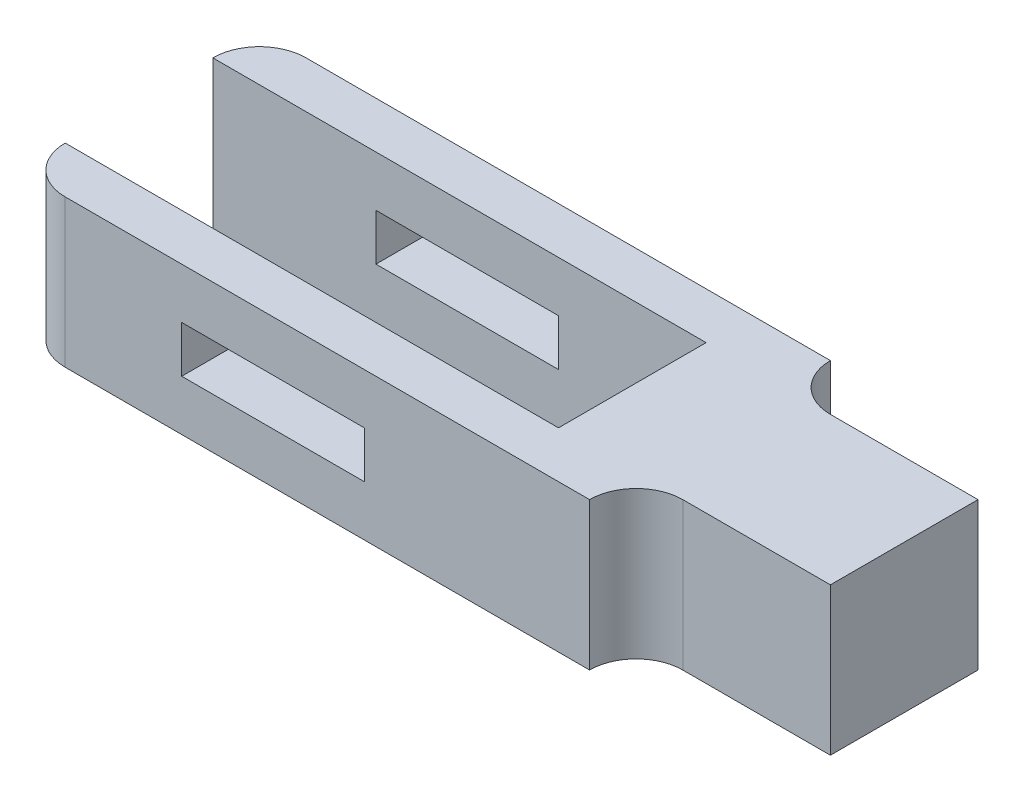
ISO-10303-21;
HEADER;
FILE_DESCRIPTION(('STEP AP214'),'2;1');
FILE_NAME('part.step','',(''),(''),'','','');
FILE_SCHEMA(('AUTOMOTIVE_DESIGN { 1 0 10303 214 1 1 1 1 }'));
ENDSEC;
DATA;
#1=APPLICATION_CONTEXT('core data for automotive mechanical design processes');
#2=APPLICATION_PROTOCOL_DEFINITION('international standard','automotive_design',2000,#1);
#3=PRODUCT_CONTEXT('',#1,'mechanical');
#4=PRODUCT('Part','Part','',(#3));
#5=PRODUCT_RELATED_PRODUCT_CATEGORY('part','',(#4));
#6=PRODUCT_DEFINITION_FORMATION('','',#4);
#7=PRODUCT_DEFINITION_CONTEXT('part definition',#1,'design');
#8=PRODUCT_DEFINITION('design','',#6,#7);
#9=PRODUCT_DEFINITION_SHAPE('','',#8);
#10=(LENGTH_UNIT() NAMED_UNIT(*) SI_UNIT(.MILLI.,.METRE.));
#11=(NAMED_UNIT(*) PLANE_ANGLE_UNIT() SI_UNIT($,.RADIAN.));
#12=(NAMED_UNIT(*) SI_UNIT($,.STERADIAN.) SOLID_ANGLE_UNIT());
#13=UNCERTAINTY_MEASURE_WITH_UNIT(LENGTH_MEASURE(1.E-05),#10,'distance_accuracy_value','');
#14=(GEOMETRIC_REPRESENTATION_CONTEXT(3) GLOBAL_UNCERTAINTY_ASSIGNED_CONTEXT((#13)) GLOBAL_UNIT_ASSIGNED_CONTEXT((#10,
#11,#12)) REPRESENTATION_CONTEXT('',''));
#15=CARTESIAN_POINT('',(0.,0.,0.));
#16=DIRECTION('',(0.,0.,1.));
#17=DIRECTION('',(1.,0.,0.));
#18=AXIS2_PLACEMENT_3D('',#15,#16,#17);
#19=CARTESIAN_POINT('',(-137.,38.,-31.));
#20=DIRECTION('',(0.,0.,1.));
#21=DIRECTION('',(1.,0.,0.));
#22=AXIS2_PLACEMENT_3D('',#19,#20,#21);
#23=PLANE('',#22);
#24=DIRECTION('',(1.,0.,0.));
#25=VECTOR('',#24,1.);
#26=CARTESIAN_POINT('',(-137.,13.,-31.));
#27=LINE('',#26,#25);
#28=CARTESIAN_POINT('',(-95.,13.,-31.));
#29=VERTEX_POINT('',#28);
#30=CARTESIAN_POINT('',(-48.,13.,-31.));
#31=VERTEX_POINT('',#30);
#32=EDGE_CURVE('E233',#29,#31,#27,.T.);
#33=ORIENTED_EDGE('',*,*,#32,.T.);
#34=DIRECTION('',(0.,1.,0.));
#35=VECTOR('',#34,1.);
#36=CARTESIAN_POINT('',(-48.,38.,-31.));
#37=LINE('',#36,#35);
#38=CARTESIAN_POINT('',(-48.,25.,-31.));
#39=VERTEX_POINT('',#38);
#40=EDGE_CURVE('E244',#31,#39,#37,.T.);
#41=ORIENTED_EDGE('',*,*,#40,.T.);
#42=DIRECTION('',(-1.,0.,0.));
#43=VECTOR('',#42,1.);
#44=CARTESIAN_POINT('',(-137.,25.,-31.));
#45=LINE('',#44,#43);
#46=CARTESIAN_POINT('',(-95.,25.,-31.));
#47=VERTEX_POINT('',#46);
#48=EDGE_CURVE('E218',#39,#47,#45,.T.);
#49=ORIENTED_EDGE('',*,*,#48,.T.);
#50=DIRECTION('',(0.,-1.,0.));
#51=VECTOR('',#50,1.);
#52=CARTESIAN_POINT('',(-95.,38.,-31.));
#53=LINE('',#52,#51);
#54=EDGE_CURVE('E227',#47,#29,#53,.T.);
#55=ORIENTED_EDGE('',*,*,#54,.T.);
#56=EDGE_LOOP('',(#33,#41,#49,#55));
#57=FACE_BOUND('',#56,.T.);
#58=DIRECTION('',(-1.,0.,0.));
#59=VECTOR('',#58,1.);
#60=CARTESIAN_POINT('',(-137.,0.,-31.));
#61=LINE('',#60,#59);
#62=CARTESIAN_POINT('',(10.,0.,-31.));
#63=VERTEX_POINT('',#62);
#64=CARTESIAN_POINT('',(-125.,0.,-31.));
#65=VERTEX_POINT('',#64);
#66=EDGE_CURVE('E268',#63,#65,#61,.T.);
#67=ORIENTED_EDGE('',*,*,#66,.T.);
#68=DIRECTION('',(0.,-1.,0.));
#69=VECTOR('',#68,1.);
#70=CARTESIAN_POINT('',(-125.,38.,-31.));
#71=LINE('',#70,#69);
#72=CARTESIAN_POINT('',(-125.,38.,-31.));
#73=VERTEX_POINT('',#72);
#74=EDGE_CURVE('E11',#65,#73,#71,.F.);
#75=ORIENTED_EDGE('',*,*,#74,.T.);
#76=DIRECTION('',(-1.,0.,0.));
#77=VECTOR('',#76,1.);
#78=CARTESIAN_POINT('',(-10.,38.,-31.));
#79=LINE('',#78,#77);
#80=CARTESIAN_POINT('',(10.,38.,-31.));
#81=VERTEX_POINT('',#80);
#82=EDGE_CURVE('E267',#81,#73,#79,.T.);
#83=ORIENTED_EDGE('',*,*,#82,.F.);
#84=DIRECTION('',(0.,-1.,0.));
#85=VECTOR('',#84,1.);
#86=CARTESIAN_POINT('',(10.,38.,-31.));
#87=LINE('',#86,#85);
#88=EDGE_CURVE('E301',#81,#63,#87,.T.);
#89=ORIENTED_EDGE('',*,*,#88,.T.);
#90=EDGE_LOOP('',(#67,#75,#83,#89));
#91=FACE_BOUND('',#90,.T.);
#92=ADVANCED_FACE('F39',(#57,#91),#23,.F.);
#93=CARTESIAN_POINT('',(-10.,38.,-19.));
#94=DIRECTION('',(0.,0.,-1.));
#95=DIRECTION('',(-1.,0.,0.));
#96=AXIS2_PLACEMENT_3D('',#93,#94,#95);
#97=PLANE('',#96);
#98=DIRECTION('',(1.,0.,0.));
#99=VECTOR('',#98,1.);
#100=CARTESIAN_POINT('',(-10.,25.,-19.));
#101=LINE('',#100,#99);
#102=CARTESIAN_POINT('',(-95.,25.,-19.));
#103=VERTEX_POINT('',#102);
#104=CARTESIAN_POINT('',(-48.,25.,-19.));
#105=VERTEX_POINT('',#104);
#106=EDGE_CURVE('E216',#103,#105,#101,.T.);
#107=ORIENTED_EDGE('',*,*,#106,.T.);
#108=DIRECTION('',(0.,-1.,0.));
#109=VECTOR('',#108,1.);
#110=CARTESIAN_POINT('',(-48.,38.,-19.));
#111=LINE('',#110,#109);
#112=CARTESIAN_POINT('',(-48.,13.,-19.));
#113=VERTEX_POINT('',#112);
#114=EDGE_CURVE('E242',#105,#113,#111,.T.);
#115=ORIENTED_EDGE('',*,*,#114,.T.);
#116=DIRECTION('',(-1.,0.,0.));
#117=VECTOR('',#116,1.);
#118=CARTESIAN_POINT('',(-10.,13.,-19.));
#119=LINE('',#118,#117);
#120=CARTESIAN_POINT('',(-95.,13.,-19.));
#121=VERTEX_POINT('',#120);
#122=EDGE_CURVE('E234',#113,#121,#119,.T.);
#123=ORIENTED_EDGE('',*,*,#122,.T.);
#124=DIRECTION('',(0.,1.,0.));
#125=VECTOR('',#124,1.);
#126=CARTESIAN_POINT('',(-95.,38.,-19.));
#127=LINE('',#126,#125);
#128=EDGE_CURVE('E224',#121,#103,#127,.T.);
#129=ORIENTED_EDGE('',*,*,#128,.T.);
#130=EDGE_LOOP('',(#107,#115,#123,#129));
#131=FACE_BOUND('',#130,.T.);
#132=DIRECTION('',(1.,0.,0.));
#133=VECTOR('',#132,1.);
#134=CARTESIAN_POINT('',(-10.,0.,-19.));
#135=LINE('',#134,#133);
#136=CARTESIAN_POINT('',(-137.,0.,-19.));
#137=VERTEX_POINT('',#136);
#138=CARTESIAN_POINT('',(-10.,0.,-19.));
#139=VERTEX_POINT('',#138);
#140=EDGE_CURVE('E285',#137,#139,#135,.T.);
#141=ORIENTED_EDGE('',*,*,#140,.T.);
#142=DIRECTION('',(0.,-1.,0.));
#143=VECTOR('',#142,1.);
#144=CARTESIAN_POINT('',(-10.,38.,-19.));
#145=LINE('',#144,#143);
#146=CARTESIAN_POINT('',(-10.,38.,-19.));
#147=VERTEX_POINT('',#146);
#148=EDGE_CURVE('E298',#147,#139,#145,.T.);
#149=ORIENTED_EDGE('',*,*,#148,.F.);
#150=DIRECTION('',(1.,0.,0.));
#151=VECTOR('',#150,1.);
#152=CARTESIAN_POINT('',(-10.,38.,-19.));
#153=LINE('',#152,#151);
#154=CARTESIAN_POINT('',(-137.,38.,-19.));
#155=VERTEX_POINT('',#154);
#156=EDGE_CURVE('E271',#155,#147,#153,.T.);
#157=ORIENTED_EDGE('',*,*,#156,.F.);
#158=DIRECTION('',(0.,-1.,0.));
#159=VECTOR('',#158,1.);
#160=CARTESIAN_POINT('',(-137.,38.,-19.));
#161=LINE('',#160,#159);
#162=EDGE_CURVE('E302',#155,#137,#161,.T.);
#163=ORIENTED_EDGE('',*,*,#162,.T.);
#164=EDGE_LOOP('',(#141,#149,#157,#163));
#165=FACE_BOUND('',#164,.T.);
#166=ADVANCED_FACE('F355',(#131,#165),#97,.F.);
#167=CARTESIAN_POINT('',(-10.,38.,19.));
#168=DIRECTION('',(1.,0.,0.));
#169=DIRECTION('',(0.,0.,-1.));
#170=AXIS2_PLACEMENT_3D('',#167,#168,#169);
#171=PLANE('',#170);
#172=DIRECTION('',(0.,0.,1.));
#173=VECTOR('',#172,1.);
#174=CARTESIAN_POINT('',(-10.,0.,19.));
#175=LINE('',#174,#173);
#176=CARTESIAN_POINT('',(-10.,0.,19.));
#177=VERTEX_POINT('',#176);
#178=EDGE_CURVE('E284',#139,#177,#175,.T.);
#179=ORIENTED_EDGE('',*,*,#178,.T.);
#180=DIRECTION('',(0.,-1.,0.));
#181=VECTOR('',#180,1.);
#182=CARTESIAN_POINT('',(-10.,38.,19.));
#183=LINE('',#182,#181);
#184=CARTESIAN_POINT('',(-10.,38.,19.));
#185=VERTEX_POINT('',#184);
#186=EDGE_CURVE('E293',#185,#177,#183,.T.);
#187=ORIENTED_EDGE('',*,*,#186,.F.);
#188=DIRECTION('',(0.,0.,1.));
#189=VECTOR('',#188,1.);
#190=CARTESIAN_POINT('',(-10.,38.,19.));
#191=LINE('',#190,#189);
#192=EDGE_CURVE('E273',#147,#185,#191,.T.);
#193=ORIENTED_EDGE('',*,*,#192,.F.);
#194=ORIENTED_EDGE('',*,*,#148,.T.);
#195=EDGE_LOOP('',(#179,#187,#193,#194));
#196=FACE_BOUND('',#195,.T.);
#197=ADVANCED_FACE('F349',(#196),#171,.F.);
#198=CARTESIAN_POINT('',(-137.,38.,19.));
#199=DIRECTION('',(0.,0.,1.));
#200=DIRECTION('',(1.,0.,0.));
#201=AXIS2_PLACEMENT_3D('',#198,#199,#200);
#202=PLANE('',#201);
#203=DIRECTION('',(1.,0.,0.));
#204=VECTOR('',#203,1.);
#205=CARTESIAN_POINT('',(-137.,13.,19.));
#206=LINE('',#205,#204);
#207=CARTESIAN_POINT('',(-95.,13.,19.));
#208=VERTEX_POINT('',#207);
#209=CARTESIAN_POINT('',(-48.,13.,19.));
#210=VERTEX_POINT('',#209);
#211=EDGE_CURVE('E229',#208,#210,#206,.T.);
#212=ORIENTED_EDGE('',*,*,#211,.T.);
#213=DIRECTION('',(0.,1.,0.));
#214=VECTOR('',#213,1.);
#215=CARTESIAN_POINT('',(-48.,38.,19.));
#216=LINE('',#215,#214);
#217=CARTESIAN_POINT('',(-48.,25.,19.));
#218=VERTEX_POINT('',#217);
#219=EDGE_CURVE('E236',#210,#218,#216,.T.);
#220=ORIENTED_EDGE('',*,*,#219,.T.);
#221=DIRECTION('',(-1.,0.,0.));
#222=VECTOR('',#221,1.);
#223=CARTESIAN_POINT('',(-137.,25.,19.));
#224=LINE('',#223,#222);
#225=CARTESIAN_POINT('',(-95.,25.,19.));
#226=VERTEX_POINT('',#225);
#227=EDGE_CURVE('E212',#218,#226,#224,.T.);
#228=ORIENTED_EDGE('',*,*,#227,.T.);
#229=DIRECTION('',(0.,-1.,0.));
#230=VECTOR('',#229,1.);
#231=CARTESIAN_POINT('',(-95.,38.,19.));
#232=LINE('',#231,#230);
#233=EDGE_CURVE('E181',#226,#208,#232,.T.);
#234=ORIENTED_EDGE('',*,*,#233,.T.);
#235=EDGE_LOOP('',(#212,#220,#228,#234));
#236=FACE_BOUND('',#235,.T.);
#237=DIRECTION('',(-1.,0.,0.));
#238=VECTOR('',#237,1.);
#239=CARTESIAN_POINT('',(-137.,0.,19.));
#240=LINE('',#239,#238);
#241=CARTESIAN_POINT('',(-137.,0.,19.));
#242=VERTEX_POINT('',#241);
#243=EDGE_CURVE('E287',#177,#242,#240,.T.);
#244=ORIENTED_EDGE('',*,*,#243,.T.);
#245=DIRECTION('',(0.,-1.,0.));
#246=VECTOR('',#245,1.);
#247=CARTESIAN_POINT('',(-137.,38.,19.));
#248=LINE('',#247,#246);
#249=CARTESIAN_POINT('',(-137.,38.,19.));
#250=VERTEX_POINT('',#249);
#251=EDGE_CURVE('E295',#250,#242,#248,.T.);
#252=ORIENTED_EDGE('',*,*,#251,.F.);
#253=DIRECTION('',(-1.,0.,0.));
#254=VECTOR('',#253,1.);
#255=CARTESIAN_POINT('',(-137.,38.,19.));
#256=LINE('',#255,#254);
#257=EDGE_CURVE('E277',#185,#250,#256,.T.);
#258=ORIENTED_EDGE('',*,*,#257,.F.);
#259=ORIENTED_EDGE('',*,*,#186,.T.);
#260=EDGE_LOOP('',(#244,#252,#258,#259));
#261=FACE_BOUND('',#260,.T.);
#262=ADVANCED_FACE('F343',(#236,#261),#202,.F.);
#263=CARTESIAN_POINT('',(-10.,38.,31.));
#264=DIRECTION('',(0.,0.,-1.));
#265=DIRECTION('',(-1.,0.,0.));
#266=AXIS2_PLACEMENT_3D('',#263,#264,#265);
#267=PLANE('',#266);
#268=DIRECTION('',(-1.,0.,0.));
#269=VECTOR('',#268,1.);
#270=CARTESIAN_POINT('',(-95.,25.,31.));
#271=LINE('',#270,#269);
#272=CARTESIAN_POINT('',(-48.,25.,31.));
#273=VERTEX_POINT('',#272);
#274=CARTESIAN_POINT('',(-95.,25.,31.));
#275=VERTEX_POINT('',#274);
#276=EDGE_CURVE('E192',#273,#275,#271,.T.);
#277=ORIENTED_EDGE('',*,*,#276,.F.);
#278=DIRECTION('',(0.,1.,0.));
#279=VECTOR('',#278,1.);
#280=CARTESIAN_POINT('',(-48.,13.,31.));
#281=LINE('',#280,#279);
#282=CARTESIAN_POINT('',(-48.,13.,31.));
#283=VERTEX_POINT('',#282);
#284=EDGE_CURVE('E197',#283,#273,#281,.T.);
#285=ORIENTED_EDGE('',*,*,#284,.F.);
#286=DIRECTION('',(1.,0.,0.));
#287=VECTOR('',#286,1.);
#288=CARTESIAN_POINT('',(-95.,13.,31.));
#289=LINE('',#288,#287);
#290=CARTESIAN_POINT('',(-95.,13.,31.));
#291=VERTEX_POINT('',#290);
#292=EDGE_CURVE('E205',#291,#283,#289,.T.);
#293=ORIENTED_EDGE('',*,*,#292,.F.);
#294=DIRECTION('',(0.,-1.,0.));
#295=VECTOR('',#294,1.);
#296=CARTESIAN_POINT('',(-95.,13.,31.));
#297=LINE('',#296,#295);
#298=EDGE_CURVE('E178',#275,#291,#297,.T.);
#299=ORIENTED_EDGE('',*,*,#298,.F.);
#300=EDGE_LOOP('',(#277,#285,#293,#299));
#301=FACE_BOUND('',#300,.T.);
#302=DIRECTION('',(1.,0.,0.));
#303=VECTOR('',#302,1.);
#304=CARTESIAN_POINT('',(-10.,38.,31.));
#305=LINE('',#304,#303);
#306=CARTESIAN_POINT('',(-125.,38.,31.));
#307=VERTEX_POINT('',#306);
#308=CARTESIAN_POINT('',(10.,38.,31.));
#309=VERTEX_POINT('',#308);
#310=EDGE_CURVE('E279',#307,#309,#305,.T.);
#311=ORIENTED_EDGE('',*,*,#310,.F.);
#312=DIRECTION('',(0.,-1.,0.));
#313=VECTOR('',#312,1.);
#314=CARTESIAN_POINT('',(-125.,38.,31.));
#315=LINE('',#314,#313);
#316=CARTESIAN_POINT('',(-125.,0.,31.));
#317=VERTEX_POINT('',#316);
#318=EDGE_CURVE('E325',#307,#317,#315,.T.);
#319=ORIENTED_EDGE('',*,*,#318,.T.);
#320=DIRECTION('',(1.,0.,0.));
#321=VECTOR('',#320,1.);
#322=CARTESIAN_POINT('',(-10.,0.,31.));
#323=LINE('',#322,#321);
#324=CARTESIAN_POINT('',(10.,0.,31.));
#325=VERTEX_POINT('',#324);
#326=EDGE_CURVE('E275',#317,#325,#323,.T.);
#327=ORIENTED_EDGE('',*,*,#326,.T.);
#328=DIRECTION('',(0.,-1.,0.));
#329=VECTOR('',#328,1.);
#330=CARTESIAN_POINT('',(10.,38.,31.));
#331=LINE('',#330,#329);
#332=EDGE_CURVE('E278',#309,#325,#331,.T.);
#333=ORIENTED_EDGE('',*,*,#332,.F.);
#334=EDGE_LOOP('',(#311,#319,#327,#333));
#335=FACE_BOUND('',#334,.T.);
#336=ADVANCED_FACE('F200',(#301,#335),#267,.F.);
#337=CARTESIAN_POINT('',(0.,38.,0.));
#338=DIRECTION('',(0.,-1.,0.));
#339=DIRECTION('',(0.,0.,-1.));
#340=AXIS2_PLACEMENT_3D('',#337,#338,#339);
#341=PLANE('',#340);
#342=ORIENTED_EDGE('',*,*,#257,.T.);
#343=CARTESIAN_POINT('',(-125.,38.,19.));
#344=DIRECTION('',(0.,-1.,0.));
#345=DIRECTION('',(0.,0.,-1.));
#346=AXIS2_PLACEMENT_3D('',#343,#344,#345);
#347=CIRCLE('',#346,12.);
#348=EDGE_CURVE('E50',#250,#307,#347,.F.);
#349=ORIENTED_EDGE('',*,*,#348,.T.);
#350=ORIENTED_EDGE('',*,*,#310,.T.);
#351=CARTESIAN_POINT('',(22.,38.,31.));
#352=DIRECTION('',(0.,-1.,0.));
#353=DIRECTION('',(0.,0.,-1.));
#354=AXIS2_PLACEMENT_3D('',#351,#352,#353);
#355=CIRCLE('',#354,12.);
#356=CARTESIAN_POINT('',(22.,38.,19.));
#357=VERTEX_POINT('',#356);
#358=EDGE_CURVE('E316',#309,#357,#355,.T.);
#359=ORIENTED_EDGE('',*,*,#358,.T.);
#360=DIRECTION('',(-1.,0.,0.));
#361=VECTOR('',#360,1.);
#362=CARTESIAN_POINT('',(60.,38.,19.));
#363=LINE('',#362,#361);
#364=CARTESIAN_POINT('',(60.,38.,19.));
#365=VERTEX_POINT('',#364);
#366=EDGE_CURVE('E265',#365,#357,#363,.T.);
#367=ORIENTED_EDGE('',*,*,#366,.F.);
#368=DIRECTION('',(0.,0.,1.));
#369=VECTOR('',#368,1.);
#370=CARTESIAN_POINT('',(60.,38.,19.));
#371=LINE('',#370,#369);
#372=CARTESIAN_POINT('',(60.,38.,-19.));
#373=VERTEX_POINT('',#372);
#374=EDGE_CURVE('E248',#373,#365,#371,.T.);
#375=ORIENTED_EDGE('',*,*,#374,.F.);
#376=DIRECTION('',(-1.,0.,0.));
#377=VECTOR('',#376,1.);
#378=CARTESIAN_POINT('',(60.,38.,-19.));
#379=LINE('',#378,#377);
#380=CARTESIAN_POINT('',(22.,38.,-19.));
#381=VERTEX_POINT('',#380);
#382=EDGE_CURVE('E264',#373,#381,#379,.T.);
#383=ORIENTED_EDGE('',*,*,#382,.T.);
#384=CARTESIAN_POINT('',(22.,38.,-31.));
#385=DIRECTION('',(0.,-1.,0.));
#386=DIRECTION('',(0.,0.,-1.));
#387=AXIS2_PLACEMENT_3D('',#384,#385,#386);
#388=CIRCLE('',#387,12.);
#389=EDGE_CURVE('E318',#381,#81,#388,.T.);
#390=ORIENTED_EDGE('',*,*,#389,.T.);
#391=ORIENTED_EDGE('',*,*,#82,.T.);
#392=CARTESIAN_POINT('',(-125.,38.,-19.));
#393=DIRECTION('',(0.,-1.,0.));
#394=DIRECTION('',(0.,0.,-1.));
#395=AXIS2_PLACEMENT_3D('',#392,#393,#394);
#396=CIRCLE('',#395,12.);
#397=EDGE_CURVE('E327',#73,#155,#396,.F.);
#398=ORIENTED_EDGE('',*,*,#397,.T.);
#399=ORIENTED_EDGE('',*,*,#156,.T.);
#400=ORIENTED_EDGE('',*,*,#192,.T.);
#401=EDGE_LOOP('',(#342,#349,#350,#359,#367,#375,#383,#390,#391,#398,#399,#400));
#402=FACE_BOUND('',#401,.T.);
#403=ADVANCED_FACE('F335',(#402),#341,.F.);
#404=CARTESIAN_POINT('',(0.,0.,0.));
#405=DIRECTION('',(0.,-1.,0.));
#406=DIRECTION('',(0.,0.,-1.));
#407=AXIS2_PLACEMENT_3D('',#404,#405,#406);
#408=PLANE('',#407);
#409=ORIENTED_EDGE('',*,*,#326,.F.);
#410=CARTESIAN_POINT('',(-125.,0.,19.));
#411=DIRECTION('',(0.,-1.,0.));
#412=DIRECTION('',(0.,0.,-1.));
#413=AXIS2_PLACEMENT_3D('',#410,#411,#412);
#414=CIRCLE('',#413,12.);
#415=EDGE_CURVE('E326',#317,#242,#414,.T.);
#416=ORIENTED_EDGE('',*,*,#415,.T.);
#417=ORIENTED_EDGE('',*,*,#243,.F.);
#418=ORIENTED_EDGE('',*,*,#178,.F.);
#419=ORIENTED_EDGE('',*,*,#140,.F.);
#420=CARTESIAN_POINT('',(-125.,0.,-19.));
#421=DIRECTION('',(0.,-1.,0.));
#422=DIRECTION('',(0.,0.,-1.));
#423=AXIS2_PLACEMENT_3D('',#420,#421,#422);
#424=CIRCLE('',#423,12.);
#425=EDGE_CURVE('E58',#137,#65,#424,.T.);
#426=ORIENTED_EDGE('',*,*,#425,.T.);
#427=ORIENTED_EDGE('',*,*,#66,.F.);
#428=CARTESIAN_POINT('',(22.,0.,-31.));
#429=DIRECTION('',(0.,-1.,0.));
#430=DIRECTION('',(0.,0.,-1.));
#431=AXIS2_PLACEMENT_3D('',#428,#429,#430);
#432=CIRCLE('',#431,12.);
#433=CARTESIAN_POINT('',(22.,0.,-19.));
#434=VERTEX_POINT('',#433);
#435=EDGE_CURVE('E319',#63,#434,#432,.F.);
#436=ORIENTED_EDGE('',*,*,#435,.T.);
#437=DIRECTION('',(-1.,0.,0.));
#438=VECTOR('',#437,1.);
#439=CARTESIAN_POINT('',(60.,0.,-19.));
#440=LINE('',#439,#438);
#441=CARTESIAN_POINT('',(60.,0.,-19.));
#442=VERTEX_POINT('',#441);
#443=EDGE_CURVE('E258',#442,#434,#440,.T.);
#444=ORIENTED_EDGE('',*,*,#443,.F.);
#445=DIRECTION('',(0.,0.,-1.));
#446=VECTOR('',#445,1.);
#447=CARTESIAN_POINT('',(60.,0.,19.));
#448=LINE('',#447,#446);
#449=CARTESIAN_POINT('',(60.,0.,19.));
#450=VERTEX_POINT('',#449);
#451=EDGE_CURVE('E255',#450,#442,#448,.T.);
#452=ORIENTED_EDGE('',*,*,#451,.F.);
#453=DIRECTION('',(-1.,0.,0.));
#454=VECTOR('',#453,1.);
#455=CARTESIAN_POINT('',(60.,0.,19.));
#456=LINE('',#455,#454);
#457=CARTESIAN_POINT('',(22.,0.,19.));
#458=VERTEX_POINT('',#457);
#459=EDGE_CURVE('E259',#450,#458,#456,.T.);
#460=ORIENTED_EDGE('',*,*,#459,.T.);
#461=CARTESIAN_POINT('',(22.,0.,31.));
#462=DIRECTION('',(0.,-1.,0.));
#463=DIRECTION('',(0.,0.,-1.));
#464=AXIS2_PLACEMENT_3D('',#461,#462,#463);
#465=CIRCLE('',#464,12.);
#466=EDGE_CURVE('E311',#458,#325,#465,.F.);
#467=ORIENTED_EDGE('',*,*,#466,.T.);
#468=EDGE_LOOP('',(#409,#416,#417,#418,#419,#426,#427,#436,#444,#452,#460,#467));
#469=FACE_BOUND('',#468,.T.);
#470=ADVANCED_FACE('F344',(#469),#408,.T.);
#471=CARTESIAN_POINT('',(60.,0.,-19.));
#472=DIRECTION('',(0.,0.,1.));
#473=DIRECTION('',(1.,0.,0.));
#474=AXIS2_PLACEMENT_3D('',#471,#472,#473);
#475=PLANE('',#474);
#476=ORIENTED_EDGE('',*,*,#443,.T.);
#477=DIRECTION('',(0.,1.,0.));
#478=VECTOR('',#477,1.);
#479=CARTESIAN_POINT('',(22.,38.,-19.));
#480=LINE('',#479,#478);
#481=EDGE_CURVE('E309',#434,#381,#480,.T.);
#482=ORIENTED_EDGE('',*,*,#481,.T.);
#483=ORIENTED_EDGE('',*,*,#382,.F.);
#484=DIRECTION('',(0.,1.,0.));
#485=VECTOR('',#484,1.);
#486=CARTESIAN_POINT('',(60.,0.,-19.));
#487=LINE('',#486,#485);
#488=EDGE_CURVE('E249',#442,#373,#487,.T.);
#489=ORIENTED_EDGE('',*,*,#488,.F.);
#490=EDGE_LOOP('',(#476,#482,#483,#489));
#491=FACE_BOUND('',#490,.T.);
#492=ADVANCED_FACE('F368',(#491),#475,.F.);
#493=CARTESIAN_POINT('',(60.,0.,19.));
#494=DIRECTION('',(0.,0.,-1.));
#495=DIRECTION('',(-1.,0.,0.));
#496=AXIS2_PLACEMENT_3D('',#493,#494,#495);
#497=PLANE('',#496);
#498=ORIENTED_EDGE('',*,*,#366,.T.);
#499=DIRECTION('',(0.,-1.,0.));
#500=VECTOR('',#499,1.);
#501=CARTESIAN_POINT('',(22.,0.,19.));
#502=LINE('',#501,#500);
#503=EDGE_CURVE('E307',#357,#458,#502,.T.);
#504=ORIENTED_EDGE('',*,*,#503,.T.);
#505=ORIENTED_EDGE('',*,*,#459,.F.);
#506=DIRECTION('',(0.,-1.,0.));
#507=VECTOR('',#506,1.);
#508=CARTESIAN_POINT('',(60.,0.,19.));
#509=LINE('',#508,#507);
#510=EDGE_CURVE('E252',#365,#450,#509,.T.);
#511=ORIENTED_EDGE('',*,*,#510,.F.);
#512=EDGE_LOOP('',(#498,#504,#505,#511));
#513=FACE_BOUND('',#512,.T.);
#514=ADVANCED_FACE('F372',(#513),#497,.F.);
#515=CARTESIAN_POINT('',(60.,0.,0.));
#516=DIRECTION('',(-1.,0.,0.));
#517=DIRECTION('',(0.,0.,1.));
#518=AXIS2_PLACEMENT_3D('',#515,#516,#517);
#519=PLANE('',#518);
#520=ORIENTED_EDGE('',*,*,#488,.T.);
#521=ORIENTED_EDGE('',*,*,#374,.T.);
#522=ORIENTED_EDGE('',*,*,#510,.T.);
#523=ORIENTED_EDGE('',*,*,#451,.T.);
#524=EDGE_LOOP('',(#520,#521,#522,#523));
#525=FACE_BOUND('',#524,.T.);
#526=ADVANCED_FACE('F369',(#525),#519,.F.);
#527=CARTESIAN_POINT('',(-95.,25.,-53.));
#528=DIRECTION('',(0.,1.,0.));
#529=DIRECTION('',(0.,0.,1.));
#530=AXIS2_PLACEMENT_3D('',#527,#528,#529);
#531=PLANE('',#530);
#532=DIRECTION('',(0.,0.,1.));
#533=VECTOR('',#532,1.);
#534=CARTESIAN_POINT('',(-48.,25.,-53.));
#535=LINE('',#534,#533);
#536=EDGE_CURVE('E191',#218,#273,#535,.T.);
#537=ORIENTED_EDGE('',*,*,#536,.T.);
#538=ORIENTED_EDGE('',*,*,#276,.T.);
#539=DIRECTION('',(0.,0.,1.));
#540=VECTOR('',#539,1.);
#541=CARTESIAN_POINT('',(-95.,25.,-53.));
#542=LINE('',#541,#540);
#543=EDGE_CURVE('E171',#226,#275,#542,.T.);
#544=ORIENTED_EDGE('',*,*,#543,.F.);
#545=ORIENTED_EDGE('',*,*,#227,.F.);
#546=EDGE_LOOP('',(#537,#538,#544,#545));
#547=FACE_BOUND('',#546,.T.);
#548=ADVANCED_FACE('F194',(#547),#531,.F.);
#549=CARTESIAN_POINT('',(-95.,13.,-53.));
#550=DIRECTION('',(-1.,0.,0.));
#551=DIRECTION('',(0.,0.,1.));
#552=AXIS2_PLACEMENT_3D('',#549,#550,#551);
#553=PLANE('',#552);
#554=ORIENTED_EDGE('',*,*,#543,.T.);
#555=ORIENTED_EDGE('',*,*,#298,.T.);
#556=DIRECTION('',(0.,0.,1.));
#557=VECTOR('',#556,1.);
#558=CARTESIAN_POINT('',(-95.,13.,-53.));
#559=LINE('',#558,#557);
#560=EDGE_CURVE('E211',#208,#291,#559,.T.);
#561=ORIENTED_EDGE('',*,*,#560,.F.);
#562=ORIENTED_EDGE('',*,*,#233,.F.);
#563=EDGE_LOOP('',(#554,#555,#561,#562));
#564=FACE_BOUND('',#563,.T.);
#565=ADVANCED_FACE('F179',(#564),#553,.F.);
#566=CARTESIAN_POINT('',(-95.,13.,-53.));
#567=DIRECTION('',(0.,-1.,0.));
#568=DIRECTION('',(0.,0.,-1.));
#569=AXIS2_PLACEMENT_3D('',#566,#567,#568);
#570=PLANE('',#569);
#571=ORIENTED_EDGE('',*,*,#560,.T.);
#572=ORIENTED_EDGE('',*,*,#292,.T.);
#573=DIRECTION('',(0.,0.,1.));
#574=VECTOR('',#573,1.);
#575=CARTESIAN_POINT('',(-48.,13.,-53.));
#576=LINE('',#575,#574);
#577=EDGE_CURVE('E210',#210,#283,#576,.T.);
#578=ORIENTED_EDGE('',*,*,#577,.F.);
#579=ORIENTED_EDGE('',*,*,#211,.F.);
#580=EDGE_LOOP('',(#571,#572,#578,#579));
#581=FACE_BOUND('',#580,.T.);
#582=ADVANCED_FACE('F426',(#581),#570,.F.);
#583=CARTESIAN_POINT('',(-48.,13.,-53.));
#584=DIRECTION('',(1.,0.,0.));
#585=DIRECTION('',(0.,0.,-1.));
#586=AXIS2_PLACEMENT_3D('',#583,#584,#585);
#587=PLANE('',#586);
#588=ORIENTED_EDGE('',*,*,#577,.T.);
#589=ORIENTED_EDGE('',*,*,#284,.T.);
#590=ORIENTED_EDGE('',*,*,#536,.F.);
#591=ORIENTED_EDGE('',*,*,#219,.F.);
#592=EDGE_LOOP('',(#588,#589,#590,#591));
#593=FACE_BOUND('',#592,.T.);
#594=ADVANCED_FACE('F416',(#593),#587,.F.);
#595=EDGE_CURVE('E207',#31,#113,#576,.T.);
#596=ORIENTED_EDGE('',*,*,#595,.T.);
#597=ORIENTED_EDGE('',*,*,#114,.F.);
#598=EDGE_CURVE('E190',#39,#105,#535,.T.);
#599=ORIENTED_EDGE('',*,*,#598,.F.);
#600=ORIENTED_EDGE('',*,*,#40,.F.);
#601=EDGE_LOOP('',(#596,#597,#599,#600));
#602=FACE_BOUND('',#601,.T.);
#603=ADVANCED_FACE('F413',(#602),#587,.F.);
#604=EDGE_CURVE('E209',#29,#121,#559,.T.);
#605=ORIENTED_EDGE('',*,*,#604,.T.);
#606=ORIENTED_EDGE('',*,*,#122,.F.);
#607=ORIENTED_EDGE('',*,*,#595,.F.);
#608=ORIENTED_EDGE('',*,*,#32,.F.);
#609=EDGE_LOOP('',(#605,#606,#607,#608));
#610=FACE_BOUND('',#609,.T.);
#611=ADVANCED_FACE('F417',(#610),#570,.F.);
#612=EDGE_CURVE('E187',#47,#103,#542,.T.);
#613=ORIENTED_EDGE('',*,*,#612,.T.);
#614=ORIENTED_EDGE('',*,*,#128,.F.);
#615=ORIENTED_EDGE('',*,*,#604,.F.);
#616=ORIENTED_EDGE('',*,*,#54,.F.);
#617=EDGE_LOOP('',(#613,#614,#615,#616));
#618=FACE_BOUND('',#617,.T.);
#619=ADVANCED_FACE('F390',(#618),#553,.F.);
#620=ORIENTED_EDGE('',*,*,#598,.T.);
#621=ORIENTED_EDGE('',*,*,#106,.F.);
#622=ORIENTED_EDGE('',*,*,#612,.F.);
#623=ORIENTED_EDGE('',*,*,#48,.F.);
#624=EDGE_LOOP('',(#620,#621,#622,#623));
#625=FACE_BOUND('',#624,.T.);
#626=ADVANCED_FACE('F377',(#625),#531,.F.);
#627=CARTESIAN_POINT('',(22.,0.,31.));
#628=DIRECTION('',(0.,1.,0.));
#629=DIRECTION('',(0.,0.,1.));
#630=AXIS2_PLACEMENT_3D('',#627,#628,#629);
#631=CYLINDRICAL_SURFACE('',#630,12.);
#632=ORIENTED_EDGE('',*,*,#358,.F.);
#633=ORIENTED_EDGE('',*,*,#332,.T.);
#634=ORIENTED_EDGE('',*,*,#466,.F.);
#635=ORIENTED_EDGE('',*,*,#503,.F.);
#636=EDGE_LOOP('',(#632,#633,#634,#635));
#637=FACE_BOUND('',#636,.T.);
#638=ADVANCED_FACE('F380',(#637),#631,.F.);
#639=CARTESIAN_POINT('',(22.,0.,-31.));
#640=DIRECTION('',(0.,-1.,0.));
#641=DIRECTION('',(0.,0.,-1.));
#642=AXIS2_PLACEMENT_3D('',#639,#640,#641);
#643=CYLINDRICAL_SURFACE('',#642,12.);
#644=ORIENTED_EDGE('',*,*,#435,.F.);
#645=ORIENTED_EDGE('',*,*,#88,.F.);
#646=ORIENTED_EDGE('',*,*,#389,.F.);
#647=ORIENTED_EDGE('',*,*,#481,.F.);
#648=EDGE_LOOP('',(#644,#645,#646,#647));
#649=FACE_BOUND('',#648,.T.);
#650=ADVANCED_FACE('F358',(#649),#643,.F.);
#651=CARTESIAN_POINT('',(-125.,38.,19.));
#652=DIRECTION('',(0.,-1.,0.));
#653=DIRECTION('',(0.,0.,-1.));
#654=AXIS2_PLACEMENT_3D('',#651,#652,#653);
#655=CYLINDRICAL_SURFACE('',#654,12.);
#656=ORIENTED_EDGE('',*,*,#348,.F.);
#657=ORIENTED_EDGE('',*,*,#251,.T.);
#658=ORIENTED_EDGE('',*,*,#415,.F.);
#659=ORIENTED_EDGE('',*,*,#318,.F.);
#660=EDGE_LOOP('',(#656,#657,#658,#659));
#661=FACE_BOUND('',#660,.T.);
#662=ADVANCED_FACE('F336',(#661),#655,.T.);
#663=CARTESIAN_POINT('',(-125.,38.,-19.));
#664=DIRECTION('',(0.,-1.,0.));
#665=DIRECTION('',(0.,0.,-1.));
#666=AXIS2_PLACEMENT_3D('',#663,#664,#665);
#667=CYLINDRICAL_SURFACE('',#666,12.);
#668=ORIENTED_EDGE('',*,*,#397,.F.);
#669=ORIENTED_EDGE('',*,*,#74,.F.);
#670=ORIENTED_EDGE('',*,*,#425,.F.);
#671=ORIENTED_EDGE('',*,*,#162,.F.);
#672=EDGE_LOOP('',(#668,#669,#670,#671));
#673=FACE_BOUND('',#672,.T.);
#674=ADVANCED_FACE('F41',(#673),#667,.T.);
#675=CLOSED_SHELL('',(#92,#166,#197,#262,#336,#403,#470,#492,#514,#526,#548,#565,#582,#594,#603,
#611,#619,#626,#638,#650,#662,#674));
#676=MANIFOLD_SOLID_BREP('B2',#675);
#677=ADVANCED_BREP_SHAPE_REPRESENTATION('',(#18,#676),#14);
#678=SHAPE_DEFINITION_REPRESENTATION(#9,#677);
ENDSEC;
END-ISO-10303-21;
